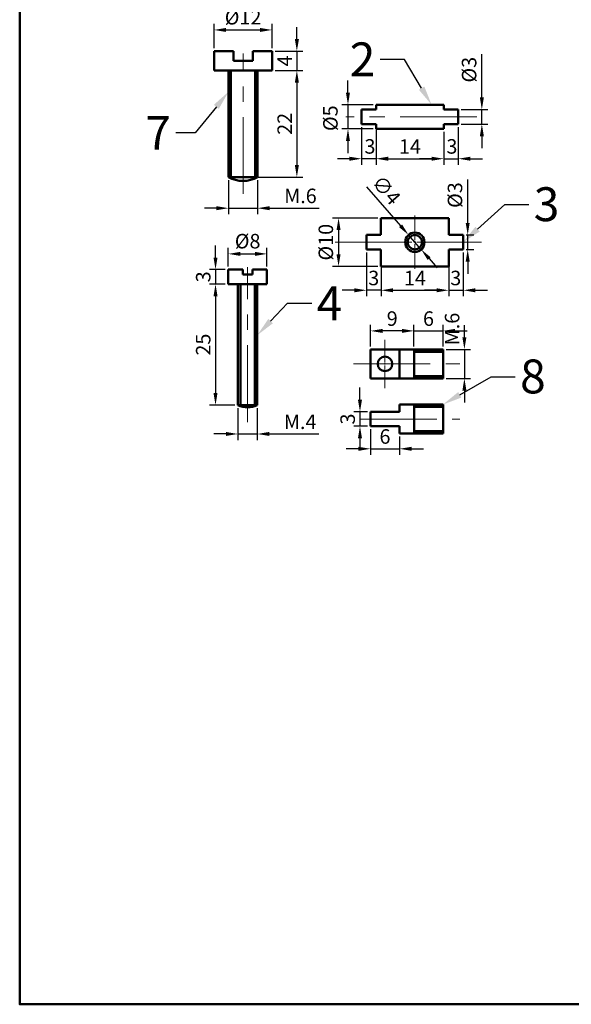
# Model space of a CAD drawing. Units: millimetres. Extents: x 77 to 718, y -35 to 313.
# Tile 1 of 7: x 77 to 191, y -35 to 169. Entities that reach past the tile are written whole.
import ezdxf
from ezdxf import colors
from ezdxf.entities.mleader import LeaderData, LeaderLine
from ezdxf.math import Vec2, Vec3

# ---------------------------------------------------------------- set-up
doc = ezdxf.new("R2010")
doc.units = ezdxf.units.MM
doc.header["$LTSCALE"] = 0.5
doc.linetypes.add('CENTER', pattern=[50.8, 31.75, -6.35, 6.35, -6.35])
for name, color, linetype, lineweight in [('M-CNTR', 1, 'CENTER', 18), ('M-DIMS', 2, 'Continuous', 25), ('M-OUTL', 7, 'Continuous', 50), ('M-TEXT', 3, 'Continuous', 25)]:
    doc.layers.add(name, color=color, linetype=linetype, lineweight=lineweight)
doc.styles.get("Standard").update_dxf_attribs({"font": 'arial.ttf'})
doc.dimstyles.new('ISO-25', dxfattribs={"dimtxt": 3, "dimasz": 2.5, "dimexe": 1.25, "dimexo": 0.625, "dimtad": 1, "dimtxsty": 'Standard', "dimcen": 2.5, "dimadec": 0, "dimazin": 0, "dimtfac": 1, "dimtmove": 0, "dimatfit": 3, "dimfxl": 1, "dimarcsym": 0})

# ---------------------------------------------------------------- blocks, each defined once
blk = doc.blocks.new('*U1')
at = {"layer": 'M-CNTR', "color": 0, "transparency": 16777216}
blk.add_line((0, -14.5), (0, 14.5), dxfattribs=at)
blk = doc.blocks.new('*D2')
at = {"layer": 'Defpoints', "color": 0, "transparency": 16777216}
for p in [(129.61, 166.47), (117.61, 162.07), (129.61, 162.07)]:
    blk.add_point(p, dxfattribs=at)
at = {"layer": 'M-DIMS', "color": 0, "lineweight": -2, "transparency": 16777216}
for p, q in [((117.61, 162.7), (117.61, 167.72)), ((129.61, 162.7), (129.61, 167.72)), ((120.11, 166.47), (127.11, 166.47))]:
    blk.add_line(p, q, dxfattribs=at)
at = {"layer": 'M-DIMS', "color": 0, "transparency": 16777216}
for points in [[(120.11, 166.89), (120.11, 166.06), (117.61, 166.47)], [(127.11, 166.89), (127.11, 166.06), (129.61, 166.47)]]:
    blk.add_solid(points, dxfattribs=at)
at = {"layer": 'M-DIMS', "color": 0, "transparency": 16777216, "insert": (123.61, 168.71), "char_height": 3, "attachment_point": 5}
blk.add_mtext('%%C12', dxfattribs=at)
blk = doc.blocks.new('*D3')
at = {"layer": 'Defpoints', "color": 0, "transparency": 16777216}
for p in [(129.61, 162.07), (129.61, 158.07), (134.74, 158.07)]:
    blk.add_point(p, dxfattribs=at)
at = {"layer": 'M-DIMS', "color": 0, "lineweight": -2, "transparency": 16777216}
for p, q in [((134.74, 164.57), (134.74, 167.07)), ((130.23, 162.07), (135.99, 162.07)), ((134.74, 162.07), (134.74, 158.07)), ((130.23, 158.07), (135.99, 158.07)), ((134.74, 155.57), (134.74, 153.07))]:
    blk.add_line(p, q, dxfattribs=at)
at = {"layer": 'M-DIMS', "color": 0, "transparency": 16777216}
for points in [[(134.32, 164.57), (135.16, 164.57), (134.74, 162.07)], [(134.32, 155.57), (135.16, 155.57), (134.74, 158.07)]]:
    blk.add_solid(points, dxfattribs=at)
at = {"layer": 'M-DIMS', "color": 0, "transparency": 16777216, "insert": (132.62, 160.07), "char_height": 3, "attachment_point": 5, "rotation": 90}
blk.add_mtext('4', dxfattribs=at)
blk = doc.blocks.new('*D4')
at = {"layer": 'Defpoints', "color": 0, "transparency": 16777216}
for p in [(129.61, 158.07), (126.11, 136.07), (134.74, 136.07)]:
    blk.add_point(p, dxfattribs=at)
at = {"layer": 'M-DIMS', "color": 0, "lineweight": -2, "transparency": 16777216}
for p, q in [((130.23, 158.07), (135.99, 158.07)), ((134.74, 155.57), (134.74, 138.57)), ((126.73, 136.07), (135.99, 136.07))]:
    blk.add_line(p, q, dxfattribs=at)
at = {"layer": 'M-DIMS', "color": 0, "transparency": 16777216}
for points in [[(134.32, 155.57), (135.16, 155.57), (134.74, 158.07)], [(134.32, 138.57), (135.16, 138.57), (134.74, 136.07)]]:
    blk.add_solid(points, dxfattribs=at)
at = {"layer": 'M-DIMS', "color": 0, "transparency": 16777216, "insert": (132.61, 147.07), "char_height": 3, "attachment_point": 5, "rotation": 90}
blk.add_mtext('22', dxfattribs=at)
blk = doc.blocks.new('*D5')
at = {"layer": 'Defpoints', "color": 0, "transparency": 16777216}
for p in [(120.61, 136.07), (126.61, 136.07), (126.61, 129.63)]:
    blk.add_point(p, dxfattribs=at)
at = {"layer": 'M-DIMS', "color": 0, "lineweight": -2, "transparency": 16777216}
for p, q in [((120.61, 135.45), (120.61, 128.38)), ((126.61, 135.45), (126.61, 128.38)), ((118.11, 129.63), (115.61, 129.63)), ((120.61, 129.63), (126.61, 129.63)), ((129.11, 129.63), (139.34, 129.63))]:
    blk.add_line(p, q, dxfattribs=at)
at = {"layer": 'M-DIMS', "color": 0, "transparency": 16777216}
for points in [[(118.11, 130.05), (118.11, 129.22), (120.61, 129.63)], [(129.11, 130.05), (129.11, 129.22), (126.61, 129.63)]]:
    blk.add_solid(points, dxfattribs=at)
at = {"layer": 'M-DIMS', "color": 0, "transparency": 16777216, "insert": (135.48, 131.79), "char_height": 3, "attachment_point": 5}
blk.add_mtext('M.6', dxfattribs=at)
blk = doc.blocks.new('*U6')
at = {"layer": 'M-CNTR', "color": 0, "transparency": 16777216}
blk.add_line((13.86, 0), (-13.26, 0), dxfattribs=at)
blk = doc.blocks.new('*D7')
at = {"layer": 'Defpoints', "color": 0, "transparency": 16777216}
for p in [(168.12, 150.01), (168.12, 147.01), (172.99, 147.01)]:
    blk.add_point(p, dxfattribs=at)
at = {"layer": 'M-DIMS', "color": 0, "lineweight": -2, "transparency": 16777216}
for p, q in [((172.99, 152.51), (172.99, 161.49)), ((168.75, 150.01), (174.24, 150.01)), ((172.99, 147.01), (172.99, 150.01)), ((168.75, 147.01), (174.24, 147.01)), ((172.99, 144.51), (172.99, 142.01))]:
    blk.add_line(p, q, dxfattribs=at)
at = {"layer": 'M-DIMS', "color": 0, "transparency": 16777216}
for points in [[(172.58, 152.51), (173.41, 152.51), (172.99, 150.01)], [(172.58, 144.51), (173.41, 144.51), (172.99, 147.01)]]:
    blk.add_solid(points, dxfattribs=at)
at = {"layer": 'M-DIMS', "color": 0, "transparency": 16777216, "insert": (170.75, 158.25), "char_height": 3, "attachment_point": 5, "rotation": 90}
blk.add_mtext('%%C3', dxfattribs=at)
blk = doc.blocks.new('*D8')
at = {"layer": 'Defpoints', "color": 0, "transparency": 16777216}
for p in [(151.12, 146.01), (165.12, 146.01), (165.12, 139.86)]:
    blk.add_point(p, dxfattribs=at)
at = {"layer": 'M-DIMS', "color": 0, "lineweight": -2, "transparency": 16777216}
for p, q in [((151.12, 145.39), (151.12, 138.61)), ((165.12, 145.39), (165.12, 138.61)), ((153.62, 139.86), (162.62, 139.86))]:
    blk.add_line(p, q, dxfattribs=at)
at = {"layer": 'M-DIMS', "color": 0, "transparency": 16777216}
for points in [[(153.62, 140.27), (153.62, 139.44), (151.12, 139.86)], [(162.62, 140.27), (162.62, 139.44), (165.12, 139.86)]]:
    blk.add_solid(points, dxfattribs=at)
at = {"layer": 'M-DIMS', "color": 0, "transparency": 16777216, "insert": (158.12, 141.99), "char_height": 3, "attachment_point": 5}
blk.add_mtext('14', dxfattribs=at)
blk = doc.blocks.new('*D9')
at = {"layer": 'Defpoints', "color": 0, "transparency": 16777216}
for p in [(168.12, 147.01), (165.12, 146.01), (168.12, 139.86)]:
    blk.add_point(p, dxfattribs=at)
at = {"layer": 'M-DIMS', "color": 0, "lineweight": -2, "transparency": 16777216}
for p, q in [((165.12, 145.39), (165.12, 138.61)), ((168.12, 146.39), (168.12, 138.61)), ((162.62, 139.86), (160.12, 139.86)), ((165.12, 139.86), (168.12, 139.86)), ((170.62, 139.86), (173.12, 139.86))]:
    blk.add_line(p, q, dxfattribs=at)
at = {"layer": 'M-DIMS', "color": 0, "transparency": 16777216}
for points in [[(162.62, 140.27), (162.62, 139.44), (165.12, 139.86)], [(170.62, 140.27), (170.62, 139.44), (168.12, 139.86)]]:
    blk.add_solid(points, dxfattribs=at)
at = {"layer": 'M-DIMS', "color": 0, "transparency": 16777216, "insert": (166.8, 142.01), "char_height": 3, "attachment_point": 5}
blk.add_mtext('3', dxfattribs=at)
blk = doc.blocks.new('*D10')
at = {"layer": 'Defpoints', "color": 0, "transparency": 16777216}
for p in [(148.12, 147.01), (151.12, 147.01), (148.12, 139.86)]:
    blk.add_point(p, dxfattribs=at)
at = {"layer": 'M-DIMS', "color": 0, "lineweight": -2, "transparency": 16777216}
for p, q in [((148.12, 146.39), (148.12, 138.61)), ((151.12, 146.39), (151.12, 138.61)), ((145.62, 139.86), (143.12, 139.86)), ((151.12, 139.86), (148.12, 139.86)), ((153.62, 139.86), (156.12, 139.86))]:
    blk.add_line(p, q, dxfattribs=at)
at = {"layer": 'M-DIMS', "color": 0, "transparency": 16777216}
for points in [[(145.62, 140.27), (145.62, 139.44), (148.12, 139.86)], [(153.62, 140.27), (153.62, 139.44), (151.12, 139.86)]]:
    blk.add_solid(points, dxfattribs=at)
at = {"layer": 'M-DIMS', "color": 0, "transparency": 16777216, "insert": (149.86, 142.01), "char_height": 3, "attachment_point": 5}
blk.add_mtext('3', dxfattribs=at)
blk = doc.blocks.new('*D11')
at = {"layer": 'Defpoints', "color": 0, "transparency": 16777216}
for p in [(151.12, 151.01), (145.31, 146.01), (151.12, 146.01)]:
    blk.add_point(p, dxfattribs=at)
at = {"layer": 'M-DIMS', "color": 0, "lineweight": -2, "transparency": 16777216}
for p, q in [((145.31, 153.51), (145.31, 156.01)), ((150.5, 151.01), (144.06, 151.01)), ((145.31, 151.01), (145.31, 146.01)), ((150.5, 146.01), (144.06, 146.01)), ((145.31, 143.51), (145.31, 141.01))]:
    blk.add_line(p, q, dxfattribs=at)
at = {"layer": 'M-DIMS', "color": 0, "transparency": 16777216}
for points in [[(144.89, 153.51), (145.72, 153.51), (145.31, 151.01)], [(144.89, 143.51), (145.72, 143.51), (145.31, 146.01)]]:
    blk.add_solid(points, dxfattribs=at)
at = {"layer": 'M-DIMS', "color": 0, "transparency": 16777216, "insert": (142.06, 148.23), "char_height": 3, "attachment_point": 5, "rotation": 90}
blk.add_mtext('%%C5', dxfattribs=at)
blk = doc.blocks.new('*U12')
at = {"layer": 'M-CNTR', "color": 0, "transparency": 16777216}
blk.add_line((0, -16), (0, 16), dxfattribs=at)
blk = doc.blocks.new('*D13')
at = {"layer": 'Defpoints', "color": 0, "transparency": 16777216}
for p in [(128.56, 120.19), (120.56, 116.94), (128.56, 116.94)]:
    blk.add_point(p, dxfattribs=at)
at = {"layer": 'M-DIMS', "color": 0, "lineweight": -2, "transparency": 16777216}
for p, q in [((120.56, 117.57), (120.56, 121.44)), ((123.06, 120.19), (126.06, 120.19)), ((128.56, 117.57), (128.56, 121.44))]:
    blk.add_line(p, q, dxfattribs=at)
at = {"layer": 'M-DIMS', "color": 0, "transparency": 16777216}
for points in [[(123.06, 120.61), (123.06, 119.77), (120.56, 120.19)], [(126.06, 120.61), (126.06, 119.77), (128.56, 120.19)]]:
    blk.add_solid(points, dxfattribs=at)
at = {"layer": 'M-DIMS', "color": 0, "transparency": 16777216, "insert": (124.56, 122.43), "char_height": 3, "attachment_point": 5}
blk.add_mtext('%%C8', dxfattribs=at)
blk = doc.blocks.new('*D14')
at = {"layer": 'Defpoints', "color": 0, "transparency": 16777216}
for p in [(120.56, 116.94), (117.92, 113.94), (120.56, 113.94)]:
    blk.add_point(p, dxfattribs=at)
at = {"layer": 'M-DIMS', "color": 0, "lineweight": -2, "transparency": 16777216}
for p, q in [((117.92, 119.44), (117.92, 121.94)), ((119.93, 116.94), (116.67, 116.94)), ((117.92, 116.94), (117.92, 113.94)), ((119.93, 113.94), (116.67, 113.94)), ((117.92, 111.44), (117.92, 108.94))]:
    blk.add_line(p, q, dxfattribs=at)
at = {"layer": 'M-DIMS', "color": 0, "transparency": 16777216}
for points in [[(117.5, 119.44), (118.33, 119.44), (117.92, 116.94)], [(117.5, 111.44), (118.33, 111.44), (117.92, 113.94)]]:
    blk.add_solid(points, dxfattribs=at)
at = {"layer": 'M-DIMS', "color": 0, "transparency": 16777216, "insert": (115.76, 115.45), "char_height": 3, "attachment_point": 5, "rotation": 90}
blk.add_mtext('3', dxfattribs=at)
blk = doc.blocks.new('*D15')
at = {"layer": 'Defpoints', "color": 0, "transparency": 16777216}
for p in [(120.56, 113.94), (117.92, 88.94), (122.56, 88.94)]:
    blk.add_point(p, dxfattribs=at)
at = {"layer": 'M-DIMS', "color": 0, "lineweight": -2, "transparency": 16777216}
for p, q in [((119.93, 113.94), (116.67, 113.94)), ((117.92, 111.44), (117.92, 91.44)), ((121.93, 88.94), (116.67, 88.94))]:
    blk.add_line(p, q, dxfattribs=at)
at = {"layer": 'M-DIMS', "color": 0, "transparency": 16777216}
for points in [[(117.5, 111.44), (118.33, 111.44), (117.92, 113.94)], [(117.5, 91.44), (118.33, 91.44), (117.92, 88.94)]]:
    blk.add_solid(points, dxfattribs=at)
at = {"layer": 'M-DIMS', "color": 0, "transparency": 16777216, "insert": (115.76, 101.44), "char_height": 3, "attachment_point": 5, "rotation": 90}
blk.add_mtext('25', dxfattribs=at)
blk = doc.blocks.new('*D16')
at = {"layer": 'Defpoints', "color": 0, "transparency": 16777216}
for p in [(122.56, 88.94), (126.56, 88.94), (126.56, 82.97)]:
    blk.add_point(p, dxfattribs=at)
at = {"layer": 'M-DIMS', "color": 0, "lineweight": -2, "transparency": 16777216}
for p, q in [((122.56, 88.32), (122.56, 81.72)), ((126.56, 88.32), (126.56, 81.72)), ((120.06, 82.97), (117.56, 82.97)), ((122.56, 82.97), (126.56, 82.97)), ((129.06, 82.97), (139.28, 82.97))]:
    blk.add_line(p, q, dxfattribs=at)
at = {"layer": 'M-DIMS', "color": 0, "transparency": 16777216}
for points in [[(120.06, 83.39), (120.06, 82.56), (122.56, 82.97)], [(129.06, 83.39), (129.06, 82.56), (126.56, 82.97)]]:
    blk.add_solid(points, dxfattribs=at)
at = {"layer": 'M-DIMS', "color": 0, "transparency": 16777216, "insert": (135.42, 85.1), "char_height": 3, "attachment_point": 5}
blk.add_mtext('M.4', dxfattribs=at)
blk = doc.blocks.new('*U17')
at = {"layer": 'M-CNTR', "color": 0, "transparency": 16777216}
for p, q in [((0, 0.4), (0, 5.5)), ((-16.5, 0), (-0.4, 0)), ((0.4, 0), (13.77, 0)), ((0, -5.5), (0, -0.4))]:
    blk.add_line(p, q, dxfattribs=at)
at = {"layer": 'M-CNTR', "color": 0, "linetype": 'Continuous', "transparency": 16777216}
for p, q in [((-0.2, 0), (0.2, 0)), ((0, -0.2), (0, 0.2))]:
    blk.add_line(p, q, dxfattribs=at)
blk = doc.blocks.new('*D18')
at = {"layer": 'Defpoints', "color": 0, "transparency": 16777216}
for p in [(169.14, 124.1), (169.14, 121.1), (170.07, 121.1)]:
    blk.add_point(p, dxfattribs=at)
at = {"layer": 'M-DIMS', "color": 0, "lineweight": -2, "transparency": 16777216}
for p, q in [((170.07, 126.6), (170.07, 135.59)), ((169.76, 124.1), (171.32, 124.1)), ((170.07, 121.1), (170.07, 124.1)), ((169.76, 121.1), (171.32, 121.1)), ((170.07, 118.6), (170.07, 116.1))]:
    blk.add_line(p, q, dxfattribs=at)
at = {"layer": 'M-DIMS', "color": 0, "transparency": 16777216}
for points in [[(169.65, 126.6), (170.48, 126.6), (170.07, 124.1)], [(169.65, 118.6), (170.48, 118.6), (170.07, 121.1)]]:
    blk.add_solid(points, dxfattribs=at)
at = {"layer": 'M-DIMS', "color": 0, "transparency": 16777216, "insert": (167.83, 132.34), "char_height": 3, "attachment_point": 5, "rotation": 90}
blk.add_mtext('%%C3', dxfattribs=at)
blk = doc.blocks.new('*D19')
at = {"layer": 'Defpoints', "color": 0, "transparency": 16777216}
for p in [(166.14, 121.1), (169.14, 121.1), (169.14, 112.67)]:
    blk.add_point(p, dxfattribs=at)
at = {"layer": 'M-DIMS', "color": 0, "lineweight": -2, "transparency": 16777216}
for p, q in [((166.14, 120.48), (166.14, 111.42)), ((169.14, 120.48), (169.14, 111.42)), ((163.64, 112.67), (161.14, 112.67)), ((166.14, 112.67), (169.14, 112.67)), ((171.64, 112.67), (174.14, 112.67))]:
    blk.add_line(p, q, dxfattribs=at)
at = {"layer": 'M-DIMS', "color": 0, "transparency": 16777216}
for points in [[(163.64, 113.08), (163.64, 112.25), (166.14, 112.67)], [(171.64, 113.08), (171.64, 112.25), (169.14, 112.67)]]:
    blk.add_solid(points, dxfattribs=at)
at = {"layer": 'M-DIMS', "color": 0, "transparency": 16777216, "insert": (167.6, 114.82), "char_height": 3, "attachment_point": 5}
blk.add_mtext('3', dxfattribs=at)
blk = doc.blocks.new('*D20')
at = {"layer": 'Defpoints', "color": 0, "transparency": 16777216}
for p in [(152.14, 117.6), (166.14, 117.6), (166.14, 112.67)]:
    blk.add_point(p, dxfattribs=at)
at = {"layer": 'M-DIMS', "color": 0, "lineweight": -2, "transparency": 16777216}
for p, q in [((152.14, 116.98), (152.14, 111.42)), ((166.14, 116.98), (166.14, 111.42)), ((154.64, 112.67), (163.64, 112.67))]:
    blk.add_line(p, q, dxfattribs=at)
at = {"layer": 'M-DIMS', "color": 0, "transparency": 16777216}
for points in [[(154.64, 113.08), (154.64, 112.25), (152.14, 112.67)], [(163.64, 113.08), (163.64, 112.25), (166.14, 112.67)]]:
    blk.add_solid(points, dxfattribs=at)
at = {"layer": 'M-DIMS', "color": 0, "transparency": 16777216, "insert": (159.14, 114.8), "char_height": 3, "attachment_point": 5}
blk.add_mtext('14', dxfattribs=at)
blk = doc.blocks.new('*D21')
at = {"layer": 'Defpoints', "color": 0, "transparency": 16777216}
for p in [(149.14, 121.1), (152.14, 121.1), (149.14, 112.67)]:
    blk.add_point(p, dxfattribs=at)
at = {"layer": 'M-DIMS', "color": 0, "lineweight": -2, "transparency": 16777216}
for p, q in [((149.14, 120.48), (149.14, 111.42)), ((152.14, 120.48), (152.14, 111.42)), ((146.64, 112.67), (144.14, 112.67)), ((152.14, 112.67), (149.14, 112.67)), ((154.64, 112.67), (157.14, 112.67))]:
    blk.add_line(p, q, dxfattribs=at)
at = {"layer": 'M-DIMS', "color": 0, "transparency": 16777216}
for points in [[(146.64, 113.08), (146.64, 112.25), (149.14, 112.67)], [(154.64, 113.08), (154.64, 112.25), (152.14, 112.67)]]:
    blk.add_solid(points, dxfattribs=at)
at = {"layer": 'M-DIMS', "color": 0, "transparency": 16777216, "insert": (150.64, 114.82), "char_height": 3, "attachment_point": 5}
blk.add_mtext('3', dxfattribs=at)
blk = doc.blocks.new('*D22')
at = {"layer": 'Defpoints', "color": 0, "transparency": 16777216}
for p in [(152.14, 127.6), (143.36, 117.6), (152.14, 117.6)]:
    blk.add_point(p, dxfattribs=at)
at = {"layer": 'M-DIMS', "color": 0, "lineweight": -2, "transparency": 16777216}
for p, q in [((151.51, 127.6), (142.11, 127.6)), ((143.36, 125.1), (143.36, 120.1)), ((151.51, 117.6), (142.11, 117.6))]:
    blk.add_line(p, q, dxfattribs=at)
at = {"layer": 'M-DIMS', "color": 0, "transparency": 16777216}
for points in [[(142.94, 125.1), (143.78, 125.1), (143.36, 127.6)], [(142.94, 120.1), (143.78, 120.1), (143.36, 117.6)]]:
    blk.add_solid(points, dxfattribs=at)
at = {"layer": 'M-DIMS', "color": 0, "transparency": 16777216, "insert": (141.12, 122.6), "char_height": 3, "attachment_point": 5, "rotation": 90}
blk.add_mtext('%%C10', dxfattribs=at)
blk = doc.blocks.new('*D23')
at = {"layer": 'Defpoints', "color": 0, "transparency": 16777216}
for p in [(157.82, 124.11), (160.45, 121.1)]:
    blk.add_point(p, dxfattribs=at)
at = {"layer": 'M-DIMS', "color": 0, "lineweight": -2, "transparency": 16777216}
for p, q in [((149.15, 134.08), (156.18, 126)), ((160.45, 121.1), (157.82, 124.11)), ((162.09, 119.21), (163.73, 117.32))]:
    blk.add_line(p, q, dxfattribs=at)
at = {"layer": 'M-DIMS', "color": 0, "transparency": 16777216}
for points in [[(156.5, 126.27), (155.87, 125.73), (157.82, 124.11)], [(162.4, 119.48), (161.78, 118.94), (160.45, 121.1)]]:
    blk.add_solid(points, dxfattribs=at)
at = {"layer": 'M-DIMS', "color": 0, "transparency": 16777216, "insert": (152.96, 133.11), "char_height": 3, "attachment_point": 5, "rotation": 311.0352}
blk.add_mtext('∅4', dxfattribs=at)
blk = doc.blocks.new('*U24')
at = {"layer": 'M-CNTR', "color": 0, "transparency": 16777216}
blk.add_line((-11, 0), (11, 0), dxfattribs=at)
blk = doc.blocks.new('*U25')
at = {"layer": 'M-CNTR', "color": 0, "transparency": 16777216}
blk.add_line((-12.67, 0), (8, 0), dxfattribs=at)
blk = doc.blocks.new('*U26')
at = {"layer": 'M-CNTR', "color": 0, "transparency": 16777216}
for p, q in [((0, 0.3), (0, 5)), ((-5, 0), (-0.3, 0)), ((0.3, 0), (5, 0)), ((0, -5), (0, -0.3))]:
    blk.add_line(p, q, dxfattribs=at)
at = {"layer": 'M-CNTR', "color": 0, "linetype": 'Continuous', "transparency": 16777216}
for p, q in [((-0.15, 0), (0.15, 0)), ((0, -0.15), (0, 0.15))]:
    blk.add_line(p, q, dxfattribs=at)
blk = doc.blocks.new('*D27')
at = {"layer": 'Defpoints', "color": 0, "transparency": 16777216}
for p in [(149.96, 87.56), (147.79, 84.56), (149.96, 84.56)]:
    blk.add_point(p, dxfattribs=at)
at = {"layer": 'M-DIMS', "color": 0, "lineweight": -2, "transparency": 16777216}
for p, q in [((147.79, 90.06), (147.79, 92.56)), ((149.34, 87.56), (146.54, 87.56)), ((147.79, 87.56), (147.79, 84.56)), ((149.34, 84.56), (146.54, 84.56)), ((147.79, 82.06), (147.79, 79.56))]:
    blk.add_line(p, q, dxfattribs=at)
at = {"layer": 'M-DIMS', "color": 0, "transparency": 16777216}
for points in [[(147.37, 90.06), (148.21, 90.06), (147.79, 87.56)], [(147.37, 82.06), (148.21, 82.06), (147.79, 84.56)]]:
    blk.add_solid(points, dxfattribs=at)
at = {"layer": 'M-DIMS', "color": 0, "transparency": 16777216, "insert": (145.63, 86.06), "char_height": 3, "attachment_point": 5, "rotation": 90}
blk.add_mtext('3', dxfattribs=at)
blk = doc.blocks.new('*D28')
at = {"layer": 'Defpoints', "color": 0, "transparency": 16777216}
for p in [(149.96, 84.56), (155.96, 83.06), (155.96, 79.91)]:
    blk.add_point(p, dxfattribs=at)
at = {"layer": 'M-DIMS', "color": 0, "lineweight": -2, "transparency": 16777216}
for p, q in [((149.96, 83.94), (149.96, 78.66)), ((155.96, 82.44), (155.96, 78.66)), ((147.46, 79.91), (144.96, 79.91)), ((149.96, 79.91), (155.96, 79.91)), ((158.46, 79.91), (160.96, 79.91))]:
    blk.add_line(p, q, dxfattribs=at)
at = {"layer": 'M-DIMS', "color": 0, "transparency": 16777216}
for points in [[(147.46, 80.32), (147.46, 79.49), (149.96, 79.91)], [(158.46, 80.32), (158.46, 79.49), (155.96, 79.91)]]:
    blk.add_solid(points, dxfattribs=at)
at = {"layer": 'M-DIMS', "color": 0, "transparency": 16777216, "insert": (152.96, 82.06), "char_height": 3, "attachment_point": 5}
blk.add_mtext('6', dxfattribs=at)
blk = doc.blocks.new('*D29')
at = {"layer": 'Defpoints', "color": 0, "transparency": 16777216}
for p in [(164.96, 100.45), (164.96, 94.45), (169.38, 94.45)]:
    blk.add_point(p, dxfattribs=at)
at = {"layer": 'M-DIMS', "color": 0, "lineweight": -2, "transparency": 16777216}
for p, q in [((169.38, 102.95), (169.38, 105.45)), ((165.59, 100.45), (170.63, 100.45)), ((169.38, 100.45), (169.38, 94.45)), ((165.59, 94.45), (170.63, 94.45)), ((169.38, 91.95), (169.38, 89.45))]:
    blk.add_line(p, q, dxfattribs=at)
at = {"layer": 'M-DIMS', "color": 0, "transparency": 16777216}
for points in [[(168.97, 102.95), (169.8, 102.95), (169.38, 100.45)], [(168.97, 91.95), (169.8, 91.95), (169.38, 94.45)]]:
    blk.add_solid(points, dxfattribs=at)
at = {"layer": 'M-DIMS', "color": 0, "transparency": 16777216, "insert": (167.23, 104.66), "char_height": 3, "attachment_point": 5, "rotation": 90}
blk.add_mtext('M.6', dxfattribs=at)
blk = doc.blocks.new('*D30')
at = {"layer": 'Defpoints', "color": 0, "transparency": 16777216}
for p in [(164.96, 104.27), (158.96, 100.45), (164.96, 100.45)]:
    blk.add_point(p, dxfattribs=at)
at = {"layer": 'M-DIMS', "color": 0, "lineweight": -2, "transparency": 16777216}
for p, q in [((156.46, 104.27), (153.96, 104.27)), ((158.96, 101.08), (158.96, 105.52)), ((158.96, 104.27), (164.96, 104.27)), ((164.96, 101.08), (164.96, 105.52)), ((167.46, 104.27), (169.96, 104.27))]:
    blk.add_line(p, q, dxfattribs=at)
at = {"layer": 'M-DIMS', "color": 0, "transparency": 16777216}
for points in [[(156.46, 104.69), (156.46, 103.86), (158.96, 104.27)], [(167.46, 104.69), (167.46, 103.86), (164.96, 104.27)]]:
    blk.add_solid(points, dxfattribs=at)
at = {"layer": 'M-DIMS', "color": 0, "transparency": 16777216, "insert": (161.96, 106.43), "char_height": 3, "attachment_point": 5}
blk.add_mtext('6', dxfattribs=at)
blk = doc.blocks.new('*D31')
at = {"layer": 'Defpoints', "color": 0, "transparency": 16777216}
for p in [(149.96, 104.27), (149.96, 100.45), (158.96, 100.45)]:
    blk.add_point(p, dxfattribs=at)
at = {"layer": 'M-DIMS', "color": 0, "lineweight": -2, "transparency": 16777216}
for p, q in [((149.96, 101.08), (149.96, 105.52)), ((156.46, 104.27), (152.46, 104.27)), ((158.96, 101.08), (158.96, 105.52))]:
    blk.add_line(p, q, dxfattribs=at)
at = {"layer": 'M-DIMS', "color": 0, "transparency": 16777216}
for points in [[(152.46, 104.69), (152.46, 103.86), (149.96, 104.27)], [(156.46, 104.69), (156.46, 103.86), (158.96, 104.27)]]:
    blk.add_solid(points, dxfattribs=at)
at = {"layer": 'M-DIMS', "color": 0, "transparency": 16777216, "insert": (154.46, 106.43), "char_height": 3, "attachment_point": 5}
blk.add_mtext('9', dxfattribs=at)

msp = doc.modelspace()

# ---------------------------------------------------------------- linework, layer by layer
at = {"layer": 'M-OUTL'}
for p, q in [((117.609, 162.071), (117.609, 158.071)), ((121.609, 162.071), (117.609, 162.071)), ((121.609, 160.071), (121.609, 162.071)), ((129.609, 162.071), (125.609, 162.071)), ((125.609, 162.071), (125.609, 160.071)), ((129.609, 158.071), (129.609, 162.071)), ((125.609, 160.071), (121.609, 160.071)), ((117.609, 158.071), (129.609, 158.071)), ((120.609, 136.071), (120.609, 158.071)), ((126.609, 158.071), (126.609, 136.071)), ((165.121, 151.014), (151.121, 151.014)), ((151.121, 151.014), (151.121, 150.014)), ((165.121, 150.014), (165.121, 151.014)), ((148.121, 150.014), (148.121, 147.014)), ((151.121, 150.014), (148.121, 150.014)), ((168.121, 150.014), (165.121, 150.014)), ((168.121, 147.014), (168.121, 150.014)), ((148.121, 147.014), (151.121, 147.014)), ((151.121, 147.014), (151.121, 146.014)), ((165.121, 146.014), (165.121, 147.014)), ((165.121, 147.014), (168.121, 147.014)), ((151.121, 146.014), (165.121, 146.014)), ((126.609, 136.071), (120.609, 136.071)), ((166.136, 127.605), (152.136, 127.605)), ((152.136, 127.605), (152.136, 124.105)), ((166.136, 124.105), (166.136, 127.605)), ((149.136, 124.105), (149.136, 121.105)), ((152.136, 124.105), (149.136, 124.105)), ((169.136, 124.105), (166.136, 124.105)), ((169.136, 121.105), (169.136, 124.105)), ((149.136, 121.105), (152.136, 121.105)), ((152.136, 121.105), (152.136, 117.605)), ((166.136, 117.605), (166.136, 121.105)), ((166.136, 121.105), (169.136, 121.105)), ((120.559, 116.942), (120.559, 113.942)), ((123.559, 116.942), (120.559, 116.942)), ((123.559, 115.942), (123.559, 116.942)), ((128.559, 116.942), (125.559, 116.942)), ((125.559, 116.942), (125.559, 115.942)), ((128.559, 113.942), (128.559, 116.942)), ((152.136, 117.605), (166.136, 117.605)), ((125.559, 115.942), (123.559, 115.942)), ((120.559, 113.942), (128.559, 113.942)), ((122.559, 88.942), (122.559, 113.942)), ((126.559, 113.942), (126.559, 88.942)), ((149.964, 100.451), (164.964, 100.451)), ((149.964, 94.451), (149.964, 100.451)), ((155.964, 94.451), (155.964, 100.451)), ((158.964, 94.451), (158.964, 100.451)), ((164.964, 100.451), (164.964, 94.451)), ((164.964, 94.451), (149.964, 94.451)), ((126.559, 88.942), (122.559, 88.942)), ((149.964, 84.562), (149.964, 87.562)), ((149.964, 87.562), (155.964, 87.562)), ((155.964, 89.062), (164.964, 89.062)), ((155.964, 87.562), (155.964, 89.062)), ((158.964, 83.062), (158.964, 89.062)), ((164.964, 89.062), (164.964, 83.062)), ((149.964, 84.562), (155.964, 84.562)), ((155.964, 83.062), (155.964, 84.562)), ((164.964, 83.062), (155.964, 83.062))]:
    msp.add_line(p, q, dxfattribs=at)
at = {"layer": 'M-OUTL', "transparency": 33554559}
for p, q in [((121.109, 136.071), (121.109, 158.071)), ((126.109, 158.071), (126.109, 136.071)), ((123.059, 88.942), (123.059, 113.942)), ((126.059, 113.942), (126.059, 88.942)), ((158.964, 99.951), (164.964, 99.951)), ((164.964, 94.951), (158.964, 94.951)), ((158.964, 88.562), (164.964, 88.562)), ((164.964, 83.562), (158.964, 83.562))]:
    msp.add_line(p, q, dxfattribs=at)
at = {"layer": 'M-OUTL', "ltscale": 0.5}
msp.add_lwpolyline([(77.418, 312.912), (718.012, 312.912), (718.012, -34.898), (77.418, -34.898)], close=True, dxfattribs=at)
at = {"layer": 'M-OUTL'}
for centre, radius in [((159.136, 122.605), 2), ((159.136, 122.605), 1.5), ((152.964, 97.451), 1.5)]:
    msp.add_circle(centre, radius, dxfattribs=at)
for centre, radius, start, end in [((123.609, 141.267), 6, 240, 300), ((124.559, 93.08), 4.596, 244.2032, 295.7968)]:
    msp.add_arc(centre, radius, start, end, dxfattribs=at)

# ---------------------------------------------------------------- block references
at = {"layer": 'M-CNTR'}
for name, p in [('*U1', (123.609, 147.071)), ('*U6', (158.121, 148.514)), ('*U17', (159.136, 122.605)), ('*U12', (124.559, 101.442)), ('*U26', (152.964, 97.451)), ('*U24', (157.464, 97.451)), ('*U25', (160.464, 86.062))]:
    msp.add_blockref(name, p, dxfattribs=at)

# ---------------------------------------------------------------- dimensions: what is measured, and where the dimension line sits
at = {"layer": 'M-DIMS'}
for base, p1, p2, text, picture, middle in [((129.609, 166.474), (117.609, 162.071), (129.609, 162.071), '%%C<>', '*D2', (123.609, 168.714)), ((126.609, 129.633), (120.609, 136.071), (126.609, 136.071), 'M.<>', '*D5', (135.476, 131.789)), ((128.559, 120.19), (120.559, 116.942), (128.559, 116.942), '%%C<>', '*D13', (124.559, 122.431)), ((126.559, 82.973), (122.559, 88.942), (126.559, 88.942), 'M.<>', '*D16', (135.42, 85.098))]:
    dim = msp.add_linear_dim(base=base, p1=p1, p2=p2, text=text, dimstyle='ISO-25', override={"dimclrd": 0, "dimclre": 0, "dimclrt": 0}, dxfattribs=at)
    dim.commit()
    dim.dimension.update_dxf_attribs({"geometry": picture, "text_midpoint": middle})
for base, p1, p2, picture, middle in [((134.741, 158.071), (129.609, 162.071), (129.609, 158.071), '*D3', (132.616, 160.071)), ((134.741, 136.071), (129.609, 158.071), (126.109, 136.071), '*D4', (132.61, 147.071)), ((117.916, 88.942), (120.559, 113.942), (122.559, 88.942), '*D15', (115.759, 101.442))]:
    dim = msp.add_linear_dim(base=base, p1=p1, p2=p2, angle=90, dimstyle='ISO-25', override={"dimclrd": 0, "dimclre": 0, "dimclrt": 0}, dxfattribs=at)
    dim.commit()
    dim.dimension.update_dxf_attribs({"geometry": picture, "text_midpoint": middle})
for base, p1, p2, text, override, picture, middle in [((172.992, 147.014), (168.121, 150.014), (168.121, 147.014), '%%C<>', {"dimclrd": 0, "dimclre": 0, "dimclrt": 0}, '*D7', (172.992, 158.254)), ((145.308, 146.014), (151.121, 151.014), (151.121, 146.014), '%%C<>', {"dimclrd": 0, "dimclre": 0, "dimclrt": 0, "dimtmove": 2}, '*D11', (142.056, 148.234)), ((170.066, 121.105), (169.136, 124.105), (169.136, 121.105), '%%C<>', {"dimclrd": 0, "dimclre": 0, "dimclrt": 0}, '*D18', (170.066, 132.345)), ((169.382, 94.451), (164.964, 100.451), (164.964, 94.451), 'M.<>', {"dimclrd": 0, "dimclre": 0, "dimclrt": 0, "dimtmove": 2}, '*D29', (167.225, 104.662))]:
    dim = msp.add_linear_dim(base=base, p1=p1, p2=p2, angle=90, text=text, dimstyle='ISO-25', override=override, dxfattribs=at)
    dim.commit()
    dim.dimension.update_dxf_attribs({"geometry": picture, "text_midpoint": middle, "dimtype": 160})
for base, p1, p2, picture, middle in [((148.121, 139.857), (151.121, 147.014), (148.121, 147.014), '*D10', (149.857, 142.015)), ((168.121, 139.857), (165.121, 146.014), (168.121, 147.014), '*D9', (166.8, 142.015)), ((149.136, 112.665), (152.136, 121.105), (149.136, 121.105), '*D21', (150.644, 114.823)), ((169.136, 112.665), (166.136, 121.105), (169.136, 121.105), '*D19', (167.597, 114.823))]:
    dim = msp.add_linear_dim(base=base, p1=p1, p2=p2, dimstyle='ISO-25', override={"dimclrd": 0, "dimclre": 0, "dimclrt": 0, "dimtmove": 2}, dxfattribs=at)
    dim.commit()
    dim.dimension.update_dxf_attribs({"geometry": picture, "text_midpoint": middle, "dimtype": 160})
for base, p1, p2, picture, middle in [((165.121, 139.857), (151.121, 146.014), (165.121, 146.014), '*D8', (158.121, 141.988)), ((166.136, 112.665), (152.136, 117.605), (166.136, 117.605), '*D20', (159.136, 114.796)), ((149.964, 104.272), (158.964, 100.451), (149.964, 100.451), '*D31', (154.464, 106.429)), ((164.964, 104.272), (158.964, 100.451), (164.964, 100.451), '*D30', (161.964, 106.429)), ((155.964, 79.907), (149.964, 84.562), (155.964, 83.062), '*D28', (152.964, 82.063))]:
    dim = msp.add_linear_dim(base=base, p1=p1, p2=p2, dimstyle='ISO-25', override={"dimclrd": 0, "dimclre": 0, "dimclrt": 0}, dxfattribs=at)
    dim.commit()
    dim.dimension.update_dxf_attribs({"geometry": picture, "text_midpoint": middle})
dim = msp.add_diameter_dim_2p(p1=(160.449, 121.096), p2=(157.823, 124.113), dimstyle='ISO-25', override={"dimclrd": 0, "dimclre": 0, "dimclrt": 0}, dxfattribs=at)
dim.commit()
dim.dimension.update_dxf_attribs({"geometry": '*D23', "text_midpoint": (151.275, 131.637), "dimtype": 163})
dim = msp.add_linear_dim(base=(143.36, 117.605), p1=(152.136, 127.605), p2=(152.136, 117.605), angle=90, text='%%C<>', dimstyle='ISO-25', override={"dimclrd": 0, "dimclre": 0, "dimclrt": 0}, dxfattribs=at)
dim.commit()
dim.dimension.update_dxf_attribs({"geometry": '*D22', "text_midpoint": (141.12, 122.605)})
for base, p1, p2, picture, middle in [((117.916, 113.942), (120.559, 116.942), (120.559, 113.942), '*D14', (115.758, 115.451)), ((147.792, 84.562), (149.964, 87.562), (149.964, 84.562), '*D27', (145.634, 86.065))]:
    dim = msp.add_linear_dim(base=base, p1=p1, p2=p2, angle=90, dimstyle='ISO-25', override={"dimclrd": 0, "dimclre": 0, "dimclrt": 0, "dimtmove": 2}, dxfattribs=at)
    dim.commit()
    dim.dimension.update_dxf_attribs({"geometry": picture, "text_midpoint": middle, "dimtype": 160})

# ---------------------------------------------------------------- leaders
at = {"layer": 'M-TEXT'}
ml = msp.add_multileader_mtext('Standard', dxfattribs=at)
ml.set_content('2', color=256)
ml.set_leader_properties()
ml.build(insert=Vec2(0, 0))
ml.multileader.update_dxf_attribs({"dogleg_length": 5})
ctx = ml.context
ctx.base_point, ctx.char_height, ctx.landing_gap_size, ctx.plane_origin = Vec3(145.337, 160.394), 7, 1, Vec3(162.595, 151.014)
ctx.text_align_type = 2
notes = []
notes.append((ctx, [(0, (1, 1, 0), (156.974, 160.394), (-1, 0), 5, [(0, [(162.595, 151.014)], 0, [])])]))
ctx.mtext.insert, ctx.mtext.alignment, ctx.mtext.flow_direction = Vec3(150.974, 163.894), 3, 5
ml = msp.add_multileader_mtext('Standard', dxfattribs=at)
ml.set_content('7', color=256)
ml.set_leader_properties()
ml.build(insert=Vec2(0, 0))
ml.multileader.update_dxf_attribs({"dogleg_length": 4})
ctx = ml.context
ctx.base_point, ctx.char_height, ctx.landing_gap_size, ctx.plane_origin = Vec3(103.173, 145.197), 7, 1, Vec3(120.609, 153.693)
ctx.text_align_type = 2
notes.append((ctx, [(0, (1, 1, 0), (113.704, 145.197), (-1, 0), 4, [(0, [(120.609, 153.693)], 0, [])])]))
ctx.mtext.insert, ctx.mtext.alignment, ctx.mtext.flow_direction = Vec3(108.704, 148.697), 3, 5
ml = msp.add_multileader_mtext('Standard', dxfattribs=at)
ml.set_content('3', color=256)
ml.set_leader_properties()
ml.build(insert=Vec2(0, 0))
ml.multileader.update_dxf_attribs({"dogleg_length": 5})
ctx = ml.context
ctx.base_point, ctx.char_height, ctx.landing_gap_size, ctx.plane_origin = Vec3(182.721, 130.395), 7, 1, Vec3(169.136, 122.605)
notes.append((ctx, [(0, (1, 1, 0), (177.721, 130.395), (1, 0), 5, [(0, [(169.136, 122.605)], 0, [])])]))
ctx.mtext.insert, ctx.mtext.flow_direction = Vec3(183.721, 133.957), 5
ml = msp.add_multileader_mtext('Standard', dxfattribs=at)
ml.set_content('4', color=256)
ml.set_leader_properties()
ml.build(insert=Vec2(0, 0))
ml.multileader.update_dxf_attribs({"dogleg_length": 5})
ctx = ml.context
ctx.base_point, ctx.char_height, ctx.landing_gap_size, ctx.plane_origin = Vec3(137.822, 109.975), 7, 1, Vec3(126.559, 103.405)
notes.append((ctx, [(0, (1, 1, 0), (132.822, 109.975), (1, 0), 5, [(0, [(126.559, 103.405)], 0, [])])]))
ctx.mtext.insert, ctx.mtext.flow_direction = Vec3(138.822, 113.475), 5
ml = msp.add_multileader_mtext('Standard', dxfattribs=at)
ml.set_content('8', color=256)
ml.set_leader_properties()
ml.build(insert=Vec2(0, 0))
ml.multileader.update_dxf_attribs({"dogleg_length": 5})
ctx = ml.context
ctx.base_point, ctx.char_height, ctx.landing_gap_size, ctx.plane_origin = Vec3(179.902, 94.8), 7, 1, Vec3(164.964, 89.062)
notes.append((ctx, [(0, (1, 1, 0), (174.902, 94.8), (1, 0), 5, [(0, [(164.964, 89.062)], 0, [])])]))
ctx.mtext.insert, ctx.mtext.flow_direction = Vec3(180.902, 98.36), 5
for ctx, leaders in notes:
    for number, flags, end, landing, length, lines in leaders:
        leader = LeaderData()
        leader.index, (leader.has_last_leader_line, leader.has_dogleg_vector, leader.attachment_direction) = number, flags
        leader.last_leader_point, leader.dogleg_vector, leader.dogleg_length = Vec3(end), Vec3(landing), length
        for number, points, colour, breaks in lines:
            line = LeaderLine()
            line.index, line.vertices, line.color, line.breaks = number, Vec3.list(points), colors.encode_raw_color(colour), breaks
            leader.lines.append(line)
        ctx.leaders.append(leader)

doc.saveas('drawing.dxf')
